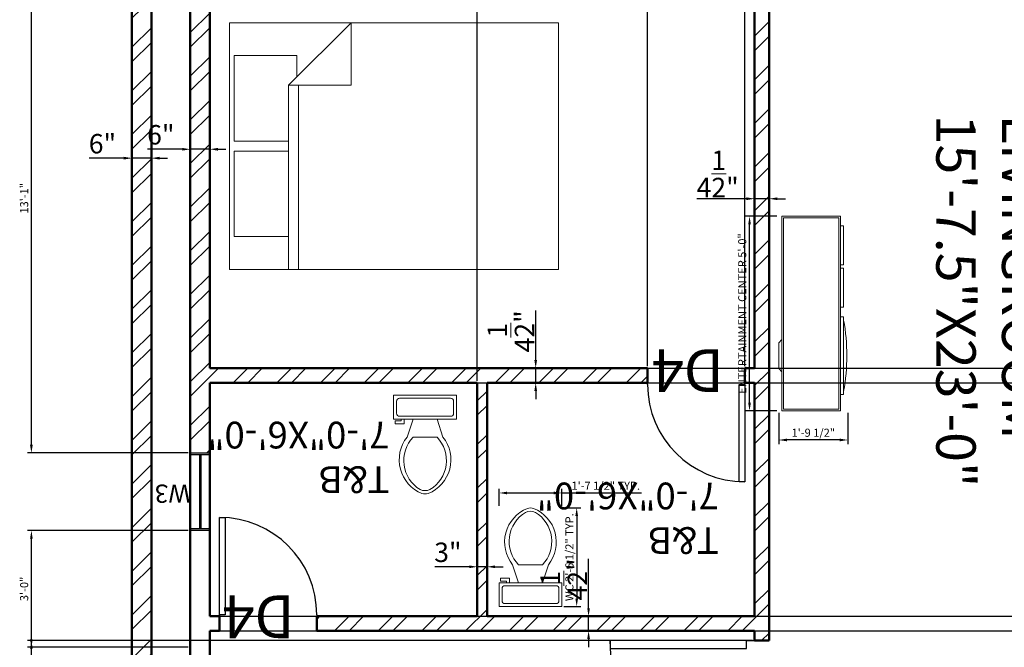
# Model space of a CAD drawing. Units: inches. Extents: x 244 to 2800, y 1060 to 1700.
# Tile 8 of 13: x 1478 to 1781, y 1287 to 1480. Entities that reach past the tile are written whole.
import ezdxf

# ---------------------------------------------------------------- set-up
doc = ezdxf.new("R2010")
doc.units = ezdxf.units.IN
for name, color, linetype, lineweight in [('A-ANNO-DIMS', 2, 'Continuous', 18), ('A-ANNO-TEXT', 1, 'Continuous', 18), ('A-DOOR', 5, 'Continuous', 25), ('A-FURN', 9, 'Continuous', 18), ('A-GLAZ', 3, 'Continuous', 25), ('A-WALL', 7, 'Continuous', 50), ('A-WALL-PATT', 8, 'Continuous', 13)]:
    doc.layers.add(name, color=color, linetype=linetype, lineweight=lineweight)
doc.styles.get("Standard").update_dxf_attribs({"font": 'arial.ttf'})
doc.dimstyles.new('ISO-25', dxfattribs={"dimtxt": 2.5, "dimasz": 2.5, "dimexe": 1.25, "dimexo": 0.625, "dimtad": 1, "dimlunit": 4, "dimtxsty": 'Standard', "dimcen": 2.5, "dimadec": 0, "dimazin": 0, "dimtfac": 1, "dimtmove": 0, "dimatfit": 3, "dimfxl": 1, "dimarcsym": 0})

# ---------------------------------------------------------------- blocks, each defined once
blk = doc.blocks.new('*U2')
for p, q in [((0, 0), (0, -5)), ((30, 0), (30, -5))]:
    blk.add_line(p, q)
blk.add_lwpolyline([(0, 0), (0, 30), (1.75, 30), (1.75, 0)], close=True)
blk.add_arc((0, 0), 30, 0, 90)
blk = doc.blocks.new('Toilet - top')
for p, q in [((9.5, -6), (9.5, -2)), ((-10, -8.5), (-8, -8.5)), ((-10, -9.5), (-10, -8.5)), ((-7, -9.5), (-10, -9.5)), ((-8, -8.5), (-8, -8)), ((-7, -8), (-7, -9.5)), ((-4, -8), (-6, -14)), ((4, -8), (6, -14)), ((4, -14), (-4, -14))]:
    blk.add_line(p, q)
blk.add_lwpolyline([(10.5, -8), (10.5, 0), (-10.5, 0), (-10.5, -8)], close=True)
for points in [[(-9.5, -2), (-9.5, -6)], [(8.5, -1), (-8.5, -1)], [(-8.5, -7), (8.5, -7)]]:
    blk.add_lwpolyline(points)
for centre, radius, start, end in [((-8.62, -1.88), 0.884, 81.8699, 188.1301), ((8.62, -1.88), 0.884, 351.8699, 98.1301), ((-8.62, -6.12), 0.884, 171.8699, 278.1301), ((8.62, -6.12), 0.884, 261.8699, 8.1301), ((3.52, -21.58), 12.17, 141.4691, 247.9714), ((4.2, -21.82), 11.33, 136.3677, 238.9468), ((-3.52, -21.58), 12.17, 292.0284, 38.5307), ((-4.2, -21.82), 11.33, 301.053, 43.6321), ((0, -27.88), 4, 245.7318, 294.2682), ((0, -29), 4, 254.8605, 285.1395)]:
    blk.add_arc(centre, radius, start, end)
blk = doc.blocks.new('Entertainment Center')
for p, q in [((-4, 0), (-5, -1)), ((4, 0), (-4, 0)), ((5, -1), (4, 0)), ((-17, -19), (-17, -1)), ((-17, -1), (43, -1)), ((-16.5, -18.5), (-16.5, -1.5)), ((-16.5, -1.5), (42.5, -1.5)), ((42.5, -1.5), (42.5, -18.5)), ((43, -1), (43, -19)), ((43, -19), (-17, -19)), ((42.5, -18.5), (-16.5, -18.5)), ((-12, -20), (-12, -19)), ((12, -20), (-12, -20)), ((12, -19), (12, -20)), ((15, -20), (15, -19)), ((27, -20), (15, -20)), ((27, -19), (27, -20)), ((28, -20), (28, -19)), ((40, -20), (28, -20)), ((40, -19), (40, -20))]:
    blk.add_line(p, q)
blk.add_arc((0, 40), 61, 259.6111, 280.3889)
blk = doc.blocks.new('Bed - Queen')
for p, q in [((0, -80.00003), (0, 0)), ((0, 0), (59.99999, 0)), ((59.99999, 0), (59.99999, -80.00003)), ((7.99999, -1.2), (28.79998, -1.2)), ((7.99999, -14.4), (7.99999, -1.2)), ((28.79998, -1.2), (28.79998, -14.4)), ((31.19999, -1.2), (51.99999, -1.2)), ((31.19999, -14.4), (31.19999, -1.2)), ((51.99999, -1.2), (51.99999, -16.4)), ((0, -14.4), (44.8, -14.4)), ((59.99999, -29.6), (44.8, -14.4)), ((44.8, -14.4), (44.8, -29.6)), ((51.99999, -16.4), (46.79936, -16.4)), ((44.8, -16.8), (0, -16.8)), ((44.8, -29.6), (59.99999, -29.6)), ((59.99999, -80.00003), (0, -80.00003))]:
    blk.add_line(p, q)
blk = doc.blocks.new('*D31')
at = {"layer": 'A-ANNO-DIMS', "color": 0, "lineweight": -2, "transparency": 16777216}
for p, q in [((1530.4, 1443.87), (1530.4, 1439.28)), ((1536.4, 1443.87), (1536.4, 1439.28)), ((1527.9, 1440.53), (1517.22, 1440.53)), ((1536.4, 1440.53), (1530.4, 1440.53)), ((1538.9, 1440.53), (1541.4, 1440.53))]:
    blk.add_line(p, q, dxfattribs=at)
at = {"layer": 'A-ANNO-DIMS', "color": 0, "transparency": 16777216}
for points in [[(1527.9, 1440.95), (1527.9, 1440.11), (1530.4, 1440.53)], [(1538.9, 1440.95), (1538.9, 1440.11), (1536.4, 1440.53)]]:
    blk.add_solid(points, dxfattribs=at)
at = {"layer": 'Defpoints', "color": 0, "transparency": 16777216}
for p in [(1530.4, 1444.49), (1536.4, 1444.49), (1530.4, 1440.53)]:
    blk.add_point(p, dxfattribs=at)
at = {"layer": 'A-ANNO-DIMS', "color": 0, "transparency": 16777216, "insert": (1521.31, 1444.22), "char_height": 6, "attachment_point": 5}
blk.add_mtext('6"', dxfattribs=at)
blk = doc.blocks.new('*D32')
at = {"layer": 'A-ANNO-DIMS', "color": 0, "lineweight": -2, "transparency": 16777216}
for p, q in [((1512.4, 1439.9), (1512.4, 1436.53)), ((1518.4, 1439.9), (1518.4, 1436.53)), ((1509.9, 1437.78), (1499.22, 1437.78)), ((1518.4, 1437.78), (1512.4, 1437.78)), ((1520.9, 1437.78), (1523.4, 1437.78))]:
    blk.add_line(p, q, dxfattribs=at)
at = {"layer": 'A-ANNO-DIMS', "color": 0, "transparency": 16777216}
for points in [[(1509.9, 1438.2), (1509.9, 1437.37), (1512.4, 1437.78)], [(1520.9, 1438.2), (1520.9, 1437.37), (1518.4, 1437.78)]]:
    blk.add_solid(points, dxfattribs=at)
at = {"layer": 'Defpoints', "color": 0, "transparency": 16777216}
for p in [(1512.4, 1440.53), (1518.4, 1440.53), (1512.4, 1437.78)]:
    blk.add_point(p, dxfattribs=at)
at = {"layer": 'A-ANNO-DIMS', "color": 0, "transparency": 16777216, "insert": (1503.31, 1441.47), "char_height": 6, "attachment_point": 5}
blk.add_mtext('6"', dxfattribs=at)
blk = doc.blocks.new('*D33')
at = {"layer": 'A-ANNO-DIMS', "color": 0, "lineweight": -2, "transparency": 16777216}
for p, q in [((1704.4, 1428.31), (1704.4, 1424.02)), ((1708.9, 1428.31), (1708.9, 1424.02)), ((1701.9, 1425.27), (1686.63, 1425.27)), ((1708.9, 1425.27), (1704.4, 1425.27)), ((1711.4, 1425.27), (1713.9, 1425.27))]:
    blk.add_line(p, q, dxfattribs=at)
at = {"layer": 'A-ANNO-DIMS', "color": 0, "transparency": 16777216}
for points in [[(1701.9, 1425.69), (1701.9, 1424.85), (1704.4, 1425.27)], [(1711.4, 1425.69), (1711.4, 1424.85), (1708.9, 1425.27)]]:
    blk.add_solid(points, dxfattribs=at)
at = {"layer": 'Defpoints', "color": 0, "transparency": 16777216}
for p in [(1704.4, 1428.93), (1708.9, 1428.93), (1704.4, 1425.27)]:
    blk.add_point(p, dxfattribs=at)
at = {"layer": 'A-ANNO-DIMS', "color": 0, "transparency": 16777216, "insert": (1693.01, 1432.92), "char_height": 6, "attachment_point": 5}
blk.add_mtext('4{\\H1x;\\S1/2;}"', dxfattribs=at)
blk = doc.blocks.new('*D34')
at = {"layer": 'A-ANNO-DIMS', "color": 0, "lineweight": -2, "transparency": 16777216}
for p, q in [((1636.9, 1375.49), (1636.9, 1390.75)), ((1634.53, 1372.99), (1638.15, 1372.99)), ((1636.9, 1368.49), (1636.9, 1372.99)), ((1634.53, 1368.49), (1638.15, 1368.49)), ((1636.9, 1365.99), (1636.9, 1363.49))]:
    blk.add_line(p, q, dxfattribs=at)
at = {"layer": 'A-ANNO-DIMS', "color": 0, "transparency": 16777216}
for points in [[(1636.48, 1375.49), (1637.31, 1375.49), (1636.9, 1372.99)], [(1636.48, 1365.99), (1637.31, 1365.99), (1636.9, 1368.49)]]:
    blk.add_solid(points, dxfattribs=at)
at = {"layer": 'Defpoints', "color": 0, "transparency": 16777216}
for p in [(1633.91, 1372.99), (1636.9, 1372.99), (1633.91, 1368.49)]:
    blk.add_point(p, dxfattribs=at)
at = {"layer": 'A-ANNO-DIMS', "color": 0, "transparency": 16777216, "insert": (1629.25, 1384.37), "char_height": 6, "attachment_point": 5, "rotation": 90}
blk.add_mtext('4{\\H1x;\\S1/2;}"', dxfattribs=at)
blk = doc.blocks.new('*D35')
at = {"layer": 'A-ANNO-DIMS', "color": 0, "lineweight": -2, "transparency": 16777216}
for p, q in [((1653.2, 1298.99), (1653.2, 1314.25)), ((1651.32, 1296.49), (1654.45, 1296.49)), ((1653.2, 1291.99), (1653.2, 1296.49)), ((1651.32, 1291.99), (1654.45, 1291.99)), ((1653.2, 1289.49), (1653.2, 1286.99))]:
    blk.add_line(p, q, dxfattribs=at)
at = {"layer": 'A-ANNO-DIMS', "color": 0, "transparency": 16777216}
for points in [[(1652.79, 1298.99), (1653.62, 1298.99), (1653.2, 1296.49)], [(1652.79, 1289.49), (1653.62, 1289.49), (1653.2, 1291.99)]]:
    blk.add_solid(points, dxfattribs=at)
at = {"layer": 'Defpoints', "color": 0, "transparency": 16777216}
for p in [(1650.7, 1296.49), (1653.2, 1296.49), (1650.7, 1291.99)]:
    blk.add_point(p, dxfattribs=at)
at = {"layer": 'A-ANNO-DIMS', "color": 0, "transparency": 16777216, "insert": (1645.55, 1307.87), "char_height": 6, "attachment_point": 5, "rotation": 90}
blk.add_mtext('4{\\H1x;\\S1/2;}"', dxfattribs=at)
blk = doc.blocks.new('*D36')
at = {"layer": 'A-ANNO-DIMS', "color": 0, "lineweight": -2, "transparency": 16777216}
for p, q in [((1618.9, 1316.15), (1618.9, 1310.51)), ((1621.9, 1316.15), (1621.9, 1310.51)), ((1616.4, 1311.76), (1605.75, 1311.76)), ((1621.9, 1311.76), (1618.9, 1311.76)), ((1624.4, 1311.76), (1626.9, 1311.76))]:
    blk.add_line(p, q, dxfattribs=at)
at = {"layer": 'A-ANNO-DIMS', "color": 0, "transparency": 16777216}
for points in [[(1616.4, 1312.18), (1616.4, 1311.34), (1618.9, 1311.76)], [(1624.4, 1312.18), (1624.4, 1311.34), (1621.9, 1311.76)]]:
    blk.add_solid(points, dxfattribs=at)
at = {"layer": 'Defpoints', "color": 0, "transparency": 16777216}
for p in [(1618.9, 1316.77), (1621.9, 1316.77), (1618.9, 1311.76)]:
    blk.add_point(p, dxfattribs=at)
at = {"layer": 'A-ANNO-DIMS', "color": 0, "transparency": 16777216, "insert": (1609.82, 1315.45), "char_height": 6, "attachment_point": 5}
blk.add_mtext('3"', dxfattribs=at)
blk = doc.blocks.new('WIN-24')
for p, q in [((0, 0), (0, 23.94)), ((0, 23.94), (6, 23.94)), ((6, 23.94), (6, 0)), ((6, 0), (0, 0))]:
    blk.add_line(p, q)
blk = doc.blocks.new('*D60')
at = {"layer": 'A-ANNO-DIMS', "color": 0, "lineweight": -2, "transparency": 16777216}
for p, q in [((1645.6, 1329.94), (1650.79, 1329.94)), ((1649.54, 1327.44), (1649.54, 1301.97)), ((1645.6, 1299.47), (1650.79, 1299.47))]:
    blk.add_line(p, q, dxfattribs=at)
at = {"layer": 'A-ANNO-DIMS', "color": 0, "transparency": 16777216}
for points in [[(1649.13, 1327.44), (1649.96, 1327.44), (1649.54, 1329.94)], [(1649.13, 1301.97), (1649.96, 1301.97), (1649.54, 1299.47)]]:
    blk.add_solid(points, dxfattribs=at)
at = {"layer": 'Defpoints', "color": 0, "transparency": 16777216}
for p in [(1644.97, 1329.94), (1644.97, 1299.47), (1649.54, 1299.47)]:
    blk.add_point(p, dxfattribs=at)
at = {"layer": 'A-ANNO-DIMS', "color": 0, "transparency": 16777216, "insert": (1647.62, 1314.71), "char_height": 2.5, "attachment_point": 5, "rotation": 90}
blk.add_mtext('WC 2\'-6 1/2" TYP.', dxfattribs=at)
blk = doc.blocks.new('*D61')
at = {"layer": 'A-ANNO-DIMS', "color": 0, "lineweight": -2, "transparency": 16777216}
for p, q in [((1625.6, 1330.57), (1625.6, 1335.77)), ((1628.1, 1334.52), (1642.47, 1334.52)), ((1644.97, 1330.57), (1644.97, 1335.77)), ((1644.97, 1334.52), (1669.55, 1334.52))]:
    blk.add_line(p, q, dxfattribs=at)
at = {"layer": 'A-ANNO-DIMS', "color": 0, "transparency": 16777216}
for points in [[(1628.1, 1334.93), (1628.1, 1334.1), (1625.6, 1334.52)], [(1642.47, 1334.93), (1642.47, 1334.1), (1644.97, 1334.52)]]:
    blk.add_solid(points, dxfattribs=at)
at = {"layer": 'Defpoints', "color": 0, "transparency": 16777216}
for p in [(1644.97, 1334.52), (1625.6, 1329.94), (1644.97, 1329.94)]:
    blk.add_point(p, dxfattribs=at)
at = {"layer": 'A-ANNO-DIMS', "color": 0, "transparency": 16777216, "insert": (1658.51, 1336.43), "char_height": 2.5, "attachment_point": 5}
blk.add_mtext('1\'-7 1/2" TYP.', dxfattribs=at)
blk = doc.blocks.new('*D70')
at = {"layer": 'A-ANNO-DIMS', "color": 0, "lineweight": -2, "transparency": 16777216}
for p, q in [((1711.21, 1419.86), (1701.59, 1419.86)), ((1702.84, 1362.36), (1702.84, 1417.36)), ((1711.21, 1359.86), (1701.59, 1359.86))]:
    blk.add_line(p, q, dxfattribs=at)
at = {"layer": 'A-ANNO-DIMS', "color": 0, "transparency": 16777216}
for points in [[(1702.42, 1417.36), (1703.25, 1417.36), (1702.84, 1419.86)], [(1702.42, 1362.36), (1703.25, 1362.36), (1702.84, 1359.86)]]:
    blk.add_solid(points, dxfattribs=at)
at = {"layer": 'Defpoints', "color": 0, "transparency": 16777216}
for p in [(1702.84, 1419.86), (1711.84, 1419.86), (1711.84, 1359.86)]:
    blk.add_point(p, dxfattribs=at)
at = {"layer": 'A-ANNO-DIMS', "color": 0, "transparency": 16777216, "insert": (1700.92, 1389.86), "char_height": 2.5, "attachment_point": 5, "rotation": 90}
blk.add_mtext('ENTERTAINMENT CENTER 5\'-0"', dxfattribs=at)
blk = doc.blocks.new('*D71')
at = {"layer": 'A-ANNO-DIMS', "color": 0, "lineweight": -2, "transparency": 16777216}
for p, q in [((1711.84, 1359.24), (1711.84, 1349.61)), ((1733.17, 1359.24), (1733.17, 1349.61)), ((1730.67, 1350.86), (1714.34, 1350.86))]:
    blk.add_line(p, q, dxfattribs=at)
at = {"layer": 'A-ANNO-DIMS', "color": 0, "transparency": 16777216}
for points in [[(1714.34, 1351.28), (1714.34, 1350.45), (1711.84, 1350.86)], [(1730.67, 1351.28), (1730.67, 1350.45), (1733.17, 1350.86)]]:
    blk.add_solid(points, dxfattribs=at)
at = {"layer": 'Defpoints', "color": 0, "transparency": 16777216}
for p in [(1711.84, 1359.86), (1733.17, 1359.86), (1711.84, 1350.86)]:
    blk.add_point(p, dxfattribs=at)
at = {"layer": 'A-ANNO-DIMS', "color": 0, "transparency": 16777216, "insert": (1722.5, 1352.78), "char_height": 2.5, "attachment_point": 5}
blk.add_mtext('1\'-9 1/2"', dxfattribs=at)
blk = doc.blocks.new('*D82')
at = {"layer": 'A-ANNO-DIMS', "color": 0, "lineweight": -2, "transparency": 16777216}
for p, q in [((1529.77, 1322.94), (1480.15, 1322.94)), ((1481.4, 1289.42), (1481.4, 1320.44)), ((1529.77, 1286.92), (1480.15, 1286.92))]:
    blk.add_line(p, q, dxfattribs=at)
at = {"layer": 'A-ANNO-DIMS', "color": 0, "transparency": 16777216}
for points in [[(1480.98, 1320.44), (1481.81, 1320.44), (1481.4, 1322.94)], [(1480.98, 1289.42), (1481.81, 1289.42), (1481.4, 1286.92)]]:
    blk.add_solid(points, dxfattribs=at)
at = {"layer": 'Defpoints', "color": 0, "transparency": 16777216}
for p in [(1481.4, 1322.94), (1530.4, 1322.94), (1530.4, 1286.92)]:
    blk.add_point(p, dxfattribs=at)
at = {"layer": 'A-ANNO-DIMS', "color": 0, "transparency": 16777216, "insert": (1479.49, 1304.93), "char_height": 2.5, "attachment_point": 5, "rotation": 90}
blk.add_mtext('3\'-0"', dxfattribs=at)
blk = doc.blocks.new('*D83')
at = {"layer": 'A-ANNO-DIMS', "color": 0, "lineweight": -2, "transparency": 16777216}
for p, q in [((1529.77, 1503.97), (1480.15, 1503.97)), ((1481.4, 1349.38), (1481.4, 1501.47)), ((1529.77, 1346.88), (1480.15, 1346.88))]:
    blk.add_line(p, q, dxfattribs=at)
at = {"layer": 'A-ANNO-DIMS', "color": 0, "transparency": 16777216}
for points in [[(1480.98, 1501.47), (1481.81, 1501.47), (1481.4, 1503.97)], [(1480.98, 1349.38), (1481.81, 1349.38), (1481.4, 1346.88)]]:
    blk.add_solid(points, dxfattribs=at)
at = {"layer": 'Defpoints', "color": 0, "transparency": 16777216}
for p in [(1481.4, 1503.97), (1530.4, 1503.97), (1530.4, 1346.88)]:
    blk.add_point(p, dxfattribs=at)
at = {"layer": 'A-ANNO-DIMS', "color": 0, "transparency": 16777216, "insert": (1479.49, 1425.42), "char_height": 2.5, "attachment_point": 5, "rotation": 90}
blk.add_mtext('13\'-1"', dxfattribs=at)
blk = doc.blocks.new('*D85')
at = {"layer": 'A-ANNO-DIMS', "color": 0, "lineweight": -2, "transparency": 16777216}
for p, q in [((1537.02, 1291.99), (2024.65, 1291.99)), ((2023.4, 1119.49), (2023.4, 1289.49)), ((1537.02, 1116.99), (2024.65, 1116.99))]:
    blk.add_line(p, q, dxfattribs=at)
at = {"layer": 'A-ANNO-DIMS', "color": 0, "transparency": 16777216}
for points in [[(2022.98, 1289.49), (2023.81, 1289.49), (2023.4, 1291.99)], [(2022.98, 1119.49), (2023.81, 1119.49), (2023.4, 1116.99)]]:
    blk.add_solid(points, dxfattribs=at)
at = {"layer": 'Defpoints', "color": 0, "transparency": 16777216}
for p in [(1536.4, 1291.99), (2023.4, 1291.99), (1536.4, 1116.99)]:
    blk.add_point(p, dxfattribs=at)
at = {"layer": 'A-ANNO-DIMS', "color": 0, "transparency": 16777216, "insert": (2021.52, 1204.49), "char_height": 2.5, "attachment_point": 5, "rotation": 90}
blk.add_mtext('14\'-7"', dxfattribs=at)
blk = doc.blocks.new('*D86')
at = {"layer": 'A-ANNO-DIMS', "color": 0, "lineweight": -2, "transparency": 16777216}
for p, q in [((1537.02, 1368.49), (2024.65, 1368.49)), ((2023.4, 1298.99), (2023.4, 1365.99)), ((1537.02, 1296.49), (2024.65, 1296.49))]:
    blk.add_line(p, q, dxfattribs=at)
at = {"layer": 'A-ANNO-DIMS', "color": 0, "transparency": 16777216}
for points in [[(2022.98, 1365.99), (2023.81, 1365.99), (2023.4, 1368.49)], [(2022.98, 1298.99), (2023.81, 1298.99), (2023.4, 1296.49)]]:
    blk.add_solid(points, dxfattribs=at)
at = {"layer": 'Defpoints', "color": 0, "transparency": 16777216}
for p in [(1536.4, 1368.49), (2023.4, 1368.49), (1536.4, 1296.49)]:
    blk.add_point(p, dxfattribs=at)
at = {"layer": 'A-ANNO-DIMS', "color": 0, "transparency": 16777216, "insert": (2021.49, 1332.49), "char_height": 2.5, "attachment_point": 5, "rotation": 90}
blk.add_mtext('6\'-0"', dxfattribs=at)
blk = doc.blocks.new('*D87')
at = {"layer": 'A-ANNO-DIMS', "color": 0, "lineweight": -2, "transparency": 16777216}
for p, q in [((1537.02, 1545.99), (2024.65, 1545.99)), ((2023.4, 1375.49), (2023.4, 1543.49)), ((1537.02, 1372.99), (2024.65, 1372.99))]:
    blk.add_line(p, q, dxfattribs=at)
at = {"layer": 'A-ANNO-DIMS', "color": 0, "transparency": 16777216}
for points in [[(2022.98, 1543.49), (2023.81, 1543.49), (2023.4, 1545.99)], [(2022.98, 1375.49), (2023.81, 1375.49), (2023.4, 1372.99)]]:
    blk.add_solid(points, dxfattribs=at)
at = {"layer": 'Defpoints', "color": 0, "transparency": 16777216}
for p in [(1536.4, 1545.99), (2023.4, 1545.99), (1536.4, 1372.99)]:
    blk.add_point(p, dxfattribs=at)
at = {"layer": 'A-ANNO-DIMS', "color": 0, "transparency": 16777216, "insert": (2021.49, 1459.49), "char_height": 2.5, "attachment_point": 5, "rotation": 90}
blk.add_mtext('14\'-5"', dxfattribs=at)
blk = doc.blocks.new('*D88')
at = {"layer": 'A-ANNO-DIMS', "color": 0, "lineweight": -2, "transparency": 16777216}
for p, q in [((1536.4, 1373.61), (1536.4, 1665.24)), ((1538.9, 1663.99), (1616.4, 1663.99)), ((1618.9, 1369.11), (1618.9, 1665.24))]:
    blk.add_line(p, q, dxfattribs=at)
at = {"layer": 'A-ANNO-DIMS', "color": 0, "transparency": 16777216}
for points in [[(1538.9, 1664.4), (1538.9, 1663.57), (1536.4, 1663.99)], [(1616.4, 1664.4), (1616.4, 1663.57), (1618.9, 1663.99)]]:
    blk.add_solid(points, dxfattribs=at)
at = {"layer": 'Defpoints', "color": 0, "transparency": 16777216}
for p in [(1618.9, 1663.99), (1536.4, 1372.99), (1618.9, 1368.49)]:
    blk.add_point(p, dxfattribs=at)
at = {"layer": 'A-ANNO-DIMS', "color": 0, "transparency": 16777216, "insert": (1577.65, 1665.9), "char_height": 2.5, "attachment_point": 5}
blk.add_mtext('6\'-10 1/2"', dxfattribs=at)
blk = doc.blocks.new('*D89')
at = {"layer": 'A-ANNO-DIMS', "color": 0, "lineweight": -2, "transparency": 16777216}
for p, q in [((1671.4, 1373.61), (1671.4, 1665.24)), ((1673.9, 1663.99), (1698.9, 1663.99)), ((1701.4, 1373.61), (1701.4, 1665.24))]:
    blk.add_line(p, q, dxfattribs=at)
at = {"layer": 'A-ANNO-DIMS', "color": 0, "transparency": 16777216}
for points in [[(1673.9, 1664.4), (1673.9, 1663.57), (1671.4, 1663.99)], [(1698.9, 1664.4), (1698.9, 1663.57), (1701.4, 1663.99)]]:
    blk.add_solid(points, dxfattribs=at)
at = {"layer": 'Defpoints', "color": 0, "transparency": 16777216}
for p in [(1701.4, 1663.99), (1671.4, 1372.99), (1701.4, 1372.99)]:
    blk.add_point(p, dxfattribs=at)
at = {"layer": 'A-ANNO-DIMS', "color": 0, "transparency": 16777216, "insert": (1686.4, 1665.89), "char_height": 2.5, "attachment_point": 5}
blk.add_mtext('2\'-6"', dxfattribs=at)
blk = doc.blocks.new('*D90')
at = {"layer": 'A-ANNO-DIMS', "color": 0, "lineweight": -2, "transparency": 16777216}
for p, q in [((1708.9, 1491.26), (1708.9, 1665.24)), ((1711.4, 1663.99), (1893.9, 1663.99)), ((1896.4, 1473.26), (1896.4, 1665.24))]:
    blk.add_line(p, q, dxfattribs=at)
at = {"layer": 'A-ANNO-DIMS', "color": 0, "transparency": 16777216}
for points in [[(1711.4, 1664.4), (1711.4, 1663.57), (1708.9, 1663.99)], [(1893.9, 1664.4), (1893.9, 1663.57), (1896.4, 1663.99)]]:
    blk.add_solid(points, dxfattribs=at)
at = {"layer": 'Defpoints', "color": 0, "transparency": 16777216}
for p in [(1896.4, 1663.99), (1708.9, 1490.64), (1896.4, 1472.64)]:
    blk.add_point(p, dxfattribs=at)
at = {"layer": 'A-ANNO-DIMS', "color": 0, "transparency": 16777216, "insert": (1802.65, 1665.9), "char_height": 2.5, "attachment_point": 5}
blk.add_mtext('15\'-7 1/2"', dxfattribs=at)
blk = doc.blocks.new('*D92')
at = {"layer": 'A-ANNO-DIMS', "color": 0, "lineweight": -2, "transparency": 16777216}
for p, q in [((1703.77, 1288.99), (1480.15, 1288.99)), ((1481.4, 1249.49), (1481.4, 1286.49)), ((1703.77, 1246.99), (1480.15, 1246.99))]:
    blk.add_line(p, q, dxfattribs=at)
at = {"layer": 'A-ANNO-DIMS', "color": 0, "transparency": 16777216}
for points in [[(1480.98, 1286.49), (1481.81, 1286.49), (1481.4, 1288.99)], [(1480.98, 1249.49), (1481.81, 1249.49), (1481.4, 1246.99)]]:
    blk.add_solid(points, dxfattribs=at)
at = {"layer": 'Defpoints', "color": 0, "transparency": 16777216}
for p in [(1481.4, 1288.99), (1704.4, 1288.99), (1704.4, 1246.99)]:
    blk.add_point(p, dxfattribs=at)
at = {"layer": 'A-ANNO-DIMS', "color": 0, "transparency": 16777216, "insert": (1479.49, 1267.99), "char_height": 2.5, "attachment_point": 5, "rotation": 90}
blk.add_mtext('3\'-6"', dxfattribs=at)

msp = doc.modelspace()

# ---------------------------------------------------------------- hatches: boundary and pattern name
at = {"layer": 'A-WALL-PATT'}
h = msp.add_hatch(dxfattribs=at)
h.set_pattern_fill('ANSI32', color=256)
h.paths.add_polyline_path([(1992.396, 1092.986), (1992.396, 1632.986), (1512.396, 1632.986), (1512.396, 1092.986)])
h.paths.add_polyline_path([(1518.396, 1098.986), (1518.396, 1626.986), (1986.396, 1626.986), (1986.396, 1098.986), (1902.396, 1098.986)], flags=16)
h.paths.add_polyline_path([(1795.896, 1110.986), (1530.396, 1110.986), (1530.396, 1551.986), (1521.7, 1551.986), (1521.7, 1623.986), (1605.7, 1623.986), (1605.7, 1551.986), (1781.396, 1551.986), (1781.396, 1545.986), (1708.896, 1545.986), (1708.896, 1532.64), (1704.396, 1532.64), (1704.396, 1545.986), (1536.396, 1545.986), (1536.396, 1372.986), (1671.396, 1372.986), (1671.396, 1368.486), (1621.896, 1368.486), (1621.896, 1296.486), (1704.396, 1296.486), (1704.396, 1368.486), (1701.396, 1368.486), (1701.396, 1372.986), (1704.396, 1372.986), (1704.396, 1490.64), (1708.896, 1490.64), (1708.896, 1288.986), (1704.396, 1288.986), (1704.396, 1291.986), (1569.396, 1291.986), (1569.396, 1296.486), (1618.896, 1296.486), (1618.896, 1368.486), (1536.396, 1368.486), (1536.396, 1296.486), (1539.396, 1296.486), (1539.396, 1291.986), (1536.396, 1291.986), (1536.396, 1116.986), (1704.396, 1116.986), (1704.396, 1246.986), (1708.896, 1246.986), (1708.896, 1116.986), (1744.896, 1116.986), (1744.896, 1260.986), (1780.896, 1260.986), (1785.396, 1260.986), (1785.396, 1205.486), (1831.896, 1205.486), (1831.896, 1217.486), (1836.396, 1217.486), (1836.396, 1205.486), (1896.396, 1205.486), (1896.396, 1265.486), (1836.396, 1265.486), (1836.396, 1253.486), (1831.896, 1253.486), (1831.896, 1269.986), (1896.396, 1269.986), (1896.396, 1472.64), (1902.396, 1472.64), (1902.396, 1242.986), (1938.396, 1242.986), (1938.396, 1134.986), (1950.396, 1134.986), (1950.396, 1242.986), (1986.396, 1242.986), (1986.396, 1134.986), (1902.396, 1134.986), (1902.396, 1110.986), (1831.896, 1110.986), (1831.896, 1116.986), (1896.396, 1116.986), (1896.396, 1200.986), (1785.396, 1200.986), (1785.396, 1116.986), (1795.896, 1116.986)], flags=0)
h.paths.add_polyline_path([(1780.896, 1116.986), (1744.896, 1116.986), (1744.896, 1260.986), (1780.896, 1260.986)], flags=0)
h.paths.add_polyline_path([(1863.351, 1110.986), (1863.351, 1116.986), (1887.296, 1116.986), (1887.296, 1110.986)], flags=0)
h.paths.add_polyline_path([(1863.851, 1114.186), (1886.796, 1114.186), (1886.796, 1113.786), (1863.851, 1113.786)], flags=0)
h.paths.add_polyline_path([(1896.396, 1174.102), (1896.396, 1198.047), (1902.396, 1198.047), (1902.396, 1174.102)], flags=0)
h.paths.add_polyline_path([(1902.396, 1174.602), (1899.196, 1174.602), (1899.196, 1197.547), (1902.396, 1197.547)], flags=0)
h.paths.add_polyline_path([(1692.519, 1110.986), (1656.574, 1110.986), (1656.574, 1116.986), (1692.519, 1116.986)], flags=0)
h.paths.add_polyline_path([(1819.776, 1376.187), (1819.776, 1410.382, -0.249194), (1838.546, 1410.382), (1838.546, 1376.187, -0.249194)], flags=0)
h.paths.add_polyline_path([(1536.396, 1250.972), (1530.396, 1250.972), (1530.396, 1286.917), (1536.396, 1286.917)], flags=0)
h.paths.add_polyline_path([(1896.396, 1405.581), (1896.396, 1453.526), (1902.396, 1453.526), (1902.396, 1405.581)], flags=0)
h.paths.add_polyline_path([(1536.396, 1322.935), (1530.396, 1322.935), (1530.396, 1346.88), (1536.396, 1346.88)], flags=0)
h.paths.add_polyline_path([(1533.196, 1323.435), (1533.196, 1346.38), (1533.596, 1346.38), (1533.596, 1323.435)], flags=0)
h.paths.add_polyline_path([(1896.396, 1545.986), (1841.396, 1545.986), (1841.396, 1551.986), (1902.396, 1551.986), (1902.396, 1532.64), (1896.396, 1532.64)], flags=0)
h.paths.add_polyline_path([(1756.808, 1545.986), (1732.863, 1545.986), (1732.863, 1551.986), (1756.808, 1551.986)], flags=0)
h.paths.add_polyline_path([(1756.308, 1548.786), (1733.363, 1548.786), (1733.363, 1551.986), (1756.308, 1551.986)], flags=0)
h.paths.add_polyline_path([(1673.743, 1545.986), (1637.798, 1545.986), (1637.798, 1551.986), (1673.743, 1551.986)], flags=0)
h.paths.add_polyline_path([(1536.396, 1503.969), (1530.396, 1503.969), (1530.396, 1539.914), (1536.396, 1539.914)], flags=0)
h.paths.add_polyline_path([(1896.341, 1192.868), (1881.737, 1192.868), (1881.737, 1181.273), (1896.341, 1181.273)], flags=8)
h.paths.add_polyline_path([(1882.893, 1112.542), (1868.29, 1112.542), (1868.29, 1100.947), (1882.893, 1100.947)], flags=8)
h.paths.add_polyline_path([(1531.898, 1340.208), (1517.295, 1340.208), (1517.295, 1328.613), (1531.898, 1328.613)], flags=24)
h.paths.add_polyline_path([(1662.207, 1564.332), (1647.603, 1564.332), (1647.603, 1552.737), (1662.207, 1552.737)], flags=8)
h.paths.add_polyline_path([(1750.605, 1565.018), (1736.001, 1565.018), (1736.001, 1553.424), (1750.605, 1553.424)], flags=8)
h.paths.add_polyline_path([(1919.351, 1440.326), (1904.748, 1440.326), (1904.748, 1428.731), (1919.351, 1428.731)], flags=8)
h.paths.add_polyline_path([(1827.662, 1149.994), (1797.512, 1149.994), (1797.512, 1122.813), (1827.662, 1122.813)], flags=8)
h.paths.add_polyline_path([(1826.683, 1247.85), (1796.533, 1247.85), (1796.533, 1220.668), (1826.683, 1220.668)], flags=8)
h.paths.add_polyline_path([(1713.043, 1285.137), (1682.893, 1285.137), (1682.893, 1257.956), (1713.043, 1257.956)], flags=8)
h.paths.add_polyline_path([(1567.301, 1310.129), (1537.151, 1310.129), (1537.151, 1282.948), (1567.301, 1282.948)], flags=8)
h.paths.add_polyline_path([(1699.655, 1386.046), (1669.505, 1386.046), (1669.505, 1358.865), (1699.655, 1358.865)], flags=8)
h.paths.add_polyline_path([(1716.254, 1527.375), (1686.103, 1527.375), (1686.103, 1500.194), (1716.254, 1500.194)], flags=8)
h.paths.add_polyline_path([(1822.088, 1577.207), (1791.938, 1577.207), (1791.938, 1550.026), (1822.088, 1550.026)], flags=8)
h.paths.add_polyline_path([(1931.716, 1518.23), (1901.565, 1518.23), (1901.565, 1491.049), (1931.716, 1491.049)], flags=8)
h.paths.add_polyline_path([(1636.272, 1573.477), (1636.272, 1615.869), (1613.819, 1615.869), (1613.819, 1573.477)], flags=8)
h.paths.add_polyline_path([(1968.141, 1266.003), (1911.144, 1266.003), (1911.144, 1252.05), (1968.141, 1252.05)], flags=8)
h.paths.add_polyline_path([(1783.26, 1275.202), (1745.711, 1275.202), (1745.711, 1261.249), (1783.26, 1261.249)], flags=8)
h.paths.add_polyline_path([(1753.522, 1456.095), (1753.522, 1338.024), (1798.876, 1338.024), (1798.876, 1456.095)], flags=8)
h.paths.add_polyline_path([(1884.04, 1192.467), (1803.345, 1192.467), (1803.345, 1149.693), (1884.04, 1149.693)], flags=8)
h.paths.add_polyline_path([(1863.426, 1264.753), (1863.426, 1209.557), (1892.661, 1209.557), (1892.661, 1264.753)], flags=8)
h.paths.add_polyline_path([(1594.411, 1361.178), (1536.688, 1361.178), (1536.688, 1330.387), (1594.411, 1330.387)], flags=8)
h.paths.add_polyline_path([(1695.984, 1342.402), (1638.262, 1342.402), (1638.262, 1311.611), (1695.984, 1311.611)], flags=8)
h.paths.add_polyline_path([(1654.435, 1540.65), (1537.752, 1540.65), (1537.752, 1489.721), (1654.435, 1489.721)], flags=8)
h.paths.add_polyline_path([(1658.864, 1271.272), (1542.182, 1271.272), (1542.182, 1220.343), (1658.864, 1220.343)], flags=8)
h = msp.add_hatch(dxfattribs=at)
h.set_pattern_fill('ANSI32', color=256)
h.paths.add_polyline_path([(1708.896, 1490.64), (1704.396, 1490.64), (1704.396, 1372.986), (1701.396, 1372.986), (1701.396, 1368.486), (1704.396, 1368.486), (1704.396, 1296.486), (1621.896, 1296.486), (1621.896, 1368.486), (1671.396, 1368.486), (1671.396, 1372.986), (1536.396, 1372.986), (1536.396, 1503.969), (1530.396, 1503.969), (1530.396, 1346.88), (1536.396, 1346.88), (1536.396, 1368.486), (1618.896, 1368.486), (1618.896, 1296.486), (1569.396, 1296.486), (1569.396, 1291.986), (1572.396, 1291.986), (1704.396, 1291.986), (1704.396, 1288.986), (1708.896, 1288.986)])

# ---------------------------------------------------------------- linework, layer by layer
at = {"layer": 'A-GLAZ'}
for p, q in [((1530.396, 1346.38), (1536.396, 1346.38)), ((1533.196, 1346.38), (1533.196, 1323.435)), ((1533.596, 1346.38), (1533.596, 1323.435)), ((1536.396, 1323.435), (1530.396, 1323.435))]:
    msp.add_line(p, q, dxfattribs=at)
at = {"layer": 'A-WALL'}
for p, q in [((1512.396, 1632.986), (1512.396, 1092.986)), ((1518.396, 1626.986), (1518.396, 1098.986)), ((1530.396, 1551.986), (1530.396, 1110.986)), ((1536.396, 1545.986), (1536.396, 1372.986)), ((1704.396, 1490.64), (1704.396, 1372.986)), ((1708.896, 1490.64), (1708.896, 1288.986)), ((1536.396, 1372.986), (1671.396, 1372.986)), ((1671.396, 1368.486), (1671.396, 1372.986)), ((1704.396, 1372.986), (1701.396, 1372.986)), ((1701.396, 1372.986), (1701.396, 1368.486)), ((1701.396, 1372.986), (1704.396, 1372.986)), ((1536.396, 1368.486), (1618.896, 1368.486)), ((1536.396, 1368.486), (1536.396, 1296.486)), ((1618.896, 1368.486), (1618.896, 1296.486)), ((1621.896, 1368.486), (1621.896, 1296.486)), ((1621.896, 1368.486), (1671.396, 1368.486)), ((1701.396, 1368.486), (1704.396, 1368.486)), ((1704.396, 1368.486), (1704.396, 1296.486)), ((1536.396, 1296.486), (1539.396, 1296.486)), ((1539.396, 1291.986), (1539.396, 1296.486)), ((1569.396, 1296.486), (1569.396, 1291.986)), ((1569.396, 1296.486), (1618.896, 1296.486)), ((1621.896, 1296.486), (1704.396, 1296.486)), ((1536.396, 1291.986), (1539.396, 1291.986)), ((1536.396, 1291.986), (1539.396, 1291.986)), ((1536.396, 1291.986), (1539.396, 1291.986)), ((1536.396, 1291.986), (1536.396, 1116.986)), ((1569.396, 1291.986), (1572.396, 1291.986)), ((1569.396, 1291.986), (1704.396, 1291.986)), ((1704.396, 1291.986), (1704.396, 1288.986)), ((1704.396, 1291.986), (1704.396, 1288.986)), ((1704.396, 1288.986), (1708.896, 1288.986))]:
    msp.add_line(p, q, dxfattribs=at)

# ---------------------------------------------------------------- block references
at = {"layer": 'A-DOOR', "rotation": 180}
msp.add_blockref('*U2', (1701.396, 1367.986), dxfattribs=at)
at = {"layer": 'A-DOOR'}
msp.add_blockref('*U2', (1539.396, 1296.986), dxfattribs=at)
at = {"layer": 'A-DOOR', "xscale": -1.399999999999999, "yscale": 1.399999999999999, "zscale": 1.399999999999999, "rotation": 90}
msp.add_blockref('*U2', (1701.896, 1288.986), dxfattribs=at)
at = {"layer": 'A-FURN'}
for name, p, xscale, yscale, zscale, rotation in [('Bed - Queen', (1542.442, 1403.45), 1.268227082860182, 1.268227082860182, 1.268227082860182, 90), ('Toilet - top', (1635.288, 1299.47), -0.9221880059424842, 0.9221880059424842, 0.9221880059424842, 180)]:
    msp.add_blockref(name, p, dxfattribs=dict(at, xscale=xscale, yscale=yscale, zscale=zscale, rotation=rotation))
at = {"layer": 'A-FURN', "rotation": 90}
msp.add_blockref('Entertainment Center', (1711.837, 1376.863), dxfattribs=at)
at = {"layer": 'A-FURN', "xscale": 0.9221880059424842, "yscale": 0.9221880059424842, "zscale": 0.9221880059424842}
msp.add_blockref('Toilet - top', (1602.783, 1364.643), dxfattribs=at)
at = {"layer": 'A-GLAZ', "rotation": 180}
msp.add_blockref('WIN-24', (1536.395, 1346.88), dxfattribs=at)

# ---------------------------------------------------------------- texts
at = {"layer": 'A-ANNO-TEXT', "attachment_point": 1}
for s, width, gutter_width, insert, char_height, rotation in [('LIVINGROOM\\P15\'-7.5"X23\'-0"', 101.44398, 60.772, (1792.837, 1451.207), 12.15447, 270), ('D4', 20.58737, 65.951, (1694.936, 1365.654), 13.1902, 180), ('T&B\\P7\'-0"X6\'-0"', 2.77063, 41.258, (1591.802, 1334.493), 8.25169, 180), ('W3', 2.91536, 28.132, (1530.396, 1331.486), 5.6265, 180), ('T&B\\P7\'-0"X6\'-0"', 2.77063, 41.258, (1693.376, 1315.717), 8.25169, 180), ('D4', 20.58737, 65.951, (1562.582, 1289.736), 13.1902, 180)]:
    msp.add_mtext_dynamic_manual_height_columns(s, width=width, gutter_width=gutter_width, heights=[0], dxfattribs=dict(at, insert=insert, char_height=char_height, rotation=rotation))

# ---------------------------------------------------------------- dimensions: what is measured, and where the dimension line sits
at = {"layer": 'A-ANNO-DIMS'}
for base, p1, p2, override, picture, middle in [((1618.896, 1663.986), (1536.396, 1372.986), (1618.896, 1368.486), {"dimdec": 1, "dimlfac": 1, "dimrnd": 0, "dimzin": 1, "dimdsep": 46, "dimlunit": 4, "dimfrac": 2}, '*D88', (1577.646, 1665.904)), ((1701.396, 1663.986), (1671.396, 1372.986), (1701.396, 1372.986), {"dimdec": 1, "dimlfac": 1, "dimrnd": 0, "dimzin": 1, "dimdsep": 46, "dimlunit": 4, "dimfrac": 2}, '*D89', (1686.396, 1665.888)), ((1896.396, 1663.986), (1708.896, 1490.64), (1896.396, 1472.64), {"dimdec": 1, "dimlfac": 1, "dimrnd": 0, "dimzin": 1, "dimdsep": 46, "dimlunit": 4, "dimfrac": 2}, '*D90', (1802.646, 1665.904)), ((1530.396, 1440.529), (1536.396, 1444.493), (1530.396, 1444.493), {"dimtxt": 6, "dimclrd": 0, "dimclre": 0, "dimclrt": 0}, '*D31', (1521.306, 1444.217)), ((1512.396, 1437.785), (1518.396, 1440.529), (1512.396, 1440.529), {"dimtxt": 6, "dimclrd": 0, "dimclre": 0, "dimclrt": 0}, '*D32', (1503.306, 1441.473)), ((1704.396, 1425.272), (1708.896, 1428.931), (1704.396, 1428.931), {"dimtxt": 6, "dimclrd": 0, "dimclre": 0, "dimclrt": 0}, '*D33', (1693.014, 1432.921)), ((1618.896, 1311.76), (1621.896, 1316.774), (1618.896, 1316.774), {"dimtxt": 6, "dimclrd": 0, "dimclre": 0, "dimclrt": 0}, '*D36', (1609.825, 1315.451))]:
    dim = msp.add_linear_dim(base=base, p1=p1, p2=p2, dimstyle='ISO-25', override=override, dxfattribs=at)
    dim.commit()
    dim.dimension.update_dxf_attribs({"geometry": picture, "text_midpoint": middle})
for base, p1, p2, angle, override, picture, middle in [((2023.396, 1545.986), (1536.396, 1372.986), (1536.396, 1545.986), 90, {"dimdec": 1, "dimlfac": 1, "dimrnd": 0, "dimzin": 1, "dimdsep": 46, "dimlunit": 4, "dimfrac": 2}, '*D87', (2021.494, 1459.486)), ((1481.396, 1503.969), (1530.396, 1346.88), (1530.396, 1503.969), 90, {"dimdec": 1, "dimlfac": 1, "dimrnd": 0, "dimzin": 1, "dimdsep": 46, "dimlunit": 4, "dimfrac": 2}, '*D83', (1479.493, 1425.425)), ((1636.898, 1372.986), (1633.907, 1368.486), (1633.907, 1372.986), 90, {"dimtxt": 6, "dimclrd": 0, "dimclre": 0, "dimclrt": 0}, '*D34', (1629.248, 1384.368)), ((2023.396, 1368.486), (1536.396, 1296.486), (1536.396, 1368.486), 90, {"dimdec": 1, "dimlfac": 1, "dimrnd": 0, "dimzin": 1, "dimdsep": 46, "dimlunit": 4, "dimfrac": 2}, '*D86', (2021.494, 1332.486)), ((1711.837, 1350.863), (1733.17, 1359.863), (1711.837, 1359.863), 180, {"dimdec": 1, "dimrnd": 0, "dimzin": 1, "dimlunit": 4, "dimfrac": 2}, '*D71', (1722.503, 1352.781)), ((1481.396, 1322.935), (1530.396, 1286.917), (1530.396, 1322.935), 90, {"dimdec": 1, "dimlfac": 1, "dimrnd": 0, "dimzin": 1, "dimdsep": 46, "dimlunit": 4, "dimfrac": 2}, '*D82', (1479.493, 1304.926)), ((1653.204, 1296.486), (1650.695, 1291.986), (1650.695, 1296.486), 90, {"dimtxt": 6, "dimclrd": 0, "dimclre": 0, "dimclrt": 0}, '*D35', (1645.554, 1307.868)), ((2023.396, 1291.986), (1536.396, 1116.986), (1536.396, 1291.986), 90, {"dimdec": 1, "dimlfac": 1, "dimrnd": 0, "dimzin": 1, "dimdsep": 46, "dimlunit": 4, "dimfrac": 2}, '*D85', (2021.516, 1204.486)), ((1481.396, 1288.986), (1704.396, 1246.986), (1704.396, 1288.986), 90, {"dimdec": 1, "dimlfac": 1, "dimrnd": 0, "dimzin": 1, "dimdsep": 46, "dimlunit": 4, "dimfrac": 2}, '*D92', (1479.493, 1267.986))]:
    dim = msp.add_linear_dim(base=base, p1=p1, p2=p2, angle=angle, dimstyle='ISO-25', override=override, dxfattribs=at)
    dim.commit()
    dim.dimension.update_dxf_attribs({"geometry": picture, "text_midpoint": middle})
for base, p1, p2, angle, text, picture, middle in [((1702.837, 1419.863), (1711.837, 1359.863), (1711.837, 1419.863), 90, 'ENTERTAINMENT CENTER <>', '*D70', (1700.919, 1389.863)), ((1649.542, 1299.47), (1644.97, 1329.945), (1644.97, 1299.47), 270, 'WC <> TYP.', '*D60', (1647.624, 1314.707))]:
    dim = msp.add_linear_dim(base=base, p1=p1, p2=p2, angle=angle, text=text, dimstyle='ISO-25', override={"dimdec": 1, "dimrnd": 0, "dimzin": 1, "dimlunit": 4, "dimfrac": 2}, dxfattribs=at)
    dim.commit()
    dim.dimension.update_dxf_attribs({"geometry": picture, "text_midpoint": middle})
dim = msp.add_linear_dim(base=(1644.97, 1334.516), p1=(1625.605, 1329.945), p2=(1644.97, 1329.945), text='<> TYP.', dimstyle='ISO-25', override={"dimdec": 1, "dimrnd": 0, "dimzin": 1, "dimlunit": 4, "dimfrac": 2}, dxfattribs=at)
dim.commit()
dim.dimension.update_dxf_attribs({"geometry": '*D61', "text_midpoint": (1658.51, 1336.434)})

doc.saveas('drawing.dxf')
